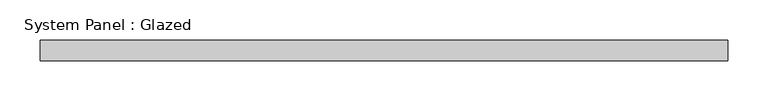
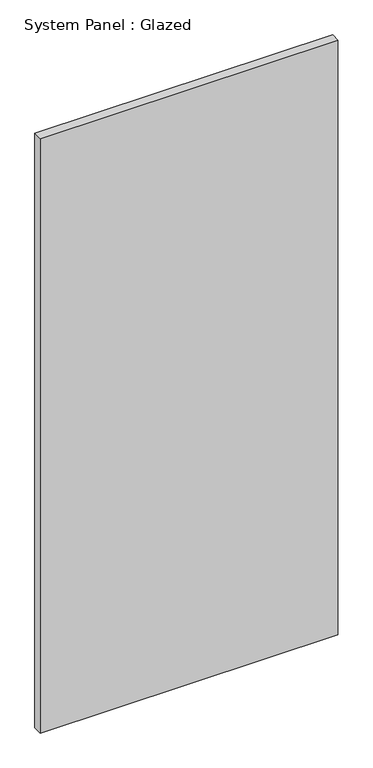
"""IFC4 building model written with IfcOpenShell, lengths in millimetres: plate geometry, System Panel : Glazed."""

from ifc_helpers import new_model, si_unit, origin, origin_with_axes, place, context, project, spatial, polyline, outline, extrude, source, transform, mapped, element, save


def system_panel_glazed_38d54ecf(model_context):
    return source(origin(), model_context, "Body", "SweptSolid", [
        extrude(outline(polyline([(425.45, 19.05), (-425.45, 19.05), (-425.45, 44.45), (425.45, 44.45), (425.45, 19.05)])), origin_with_axes(), (0.0, 0.0, 1.0), 1797.05),
    ])


if __name__ == "__main__":
    model = new_model("IFC4")
    model_context = context("Model", 3, world=origin())
    ifc_project = project(units=[si_unit("LENGTHUNIT", "METRE", prefix="MILLI")], contexts=[model_context])
    site = spatial("IfcSite", under=ifc_project)
    building = spatial("IfcBuilding", under=site)
    placement = place(None, origin())
    system_panel_glazed_shape = system_panel_glazed_38d54ecf(model_context)
    element("IfcPlate", 1, ObjectType="System Panel : Glazed", at=placement, inside=building, context=model_context, shape_type="MappedRepresentation", body=[
        mapped(system_panel_glazed_shape, transform((0.0, 0.0, 0.0), x_axis=(1.0, 0.0, 0.0), y_axis=(0.0, 1.0, 0.0), z_axis=(0.0, 0.0, 1.0))),
    ])
    save(model, "model.ifc")

# Revit data of these elements
# Type "System Panel : Glazed"
#   Construction Type Id = "GSP4R"
#   Analytic Construction = "1/8 in Pilkington single glazing"
#   Visual Light Transmittance = 0.9
#   Solar Heat Gain Coefficient = 0.86
#   Heat Transfer Coefficient (U) = 6.7069 W/(m²·K)
# Element 1 (IfcPlate, "System Panel : Glazed")
#   Materials on its faces: "Glass"
# Materials
#   "Glass": class "Glass", colour RGB 0 128 192, transparency 0.75, Description = "Soda Lime Glass", Cost = 0
